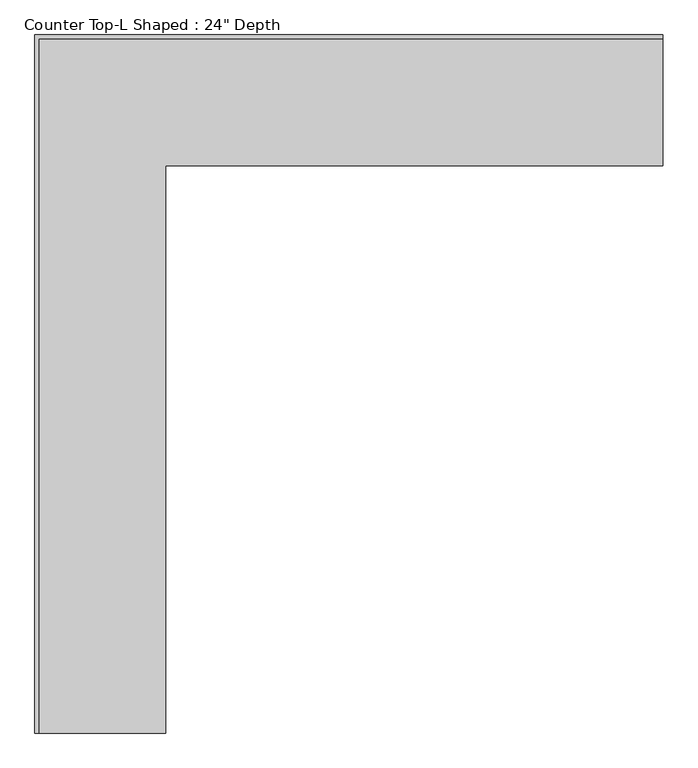
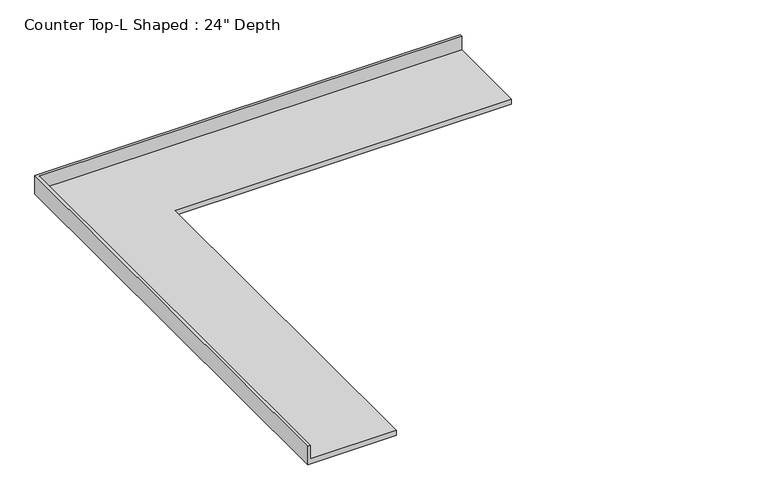
"""IFC4 building model written with IfcOpenShell, lengths in millimetres: furniture geometry."""

from ifc_helpers import new_model, si_unit, origin, place, context, project, spatial, faceted_brep, source, transform, mapped, element, save


def furniture_2797bbf7(model_context):
    return source(origin(), model_context, "Body", "Brep", [
        faceted_brep([(-565.4622951, -3387.4293744, 914.4), (-565.4622951, -635.0, 914.4), (1847.5377049, -635.0, 914.4), (1847.5377049, -19.05, 914.4), (-1181.4122951, -19.05, 914.4), (-1181.4122951, -3387.4293744, 914.4), (1847.5377049, 0.0, 876.3), (1847.5377049, -635.0, 876.3), (-565.4622951, -635.0, 876.3), (-565.4622951, -3387.4293744, 876.3), (-1200.4622951, -3387.4293744, 876.3), (-1200.4622951, 0.0, 876.3), (-1200.4622951, 0.0, 1016.0), (1847.5377049, 0.0, 1016.0), (-1200.4622951, -3387.4293744, 1016.0), (-1181.4122951, -3387.4293744, 1016.0), (1847.5377049, -19.05, 1016.0), (-1181.4122951, -19.05, 1016.0)], [[[0, 1, 2, 3, 4, 5]], [[6, 7, 8, 9, 10, 11]], [[6, 11, 12, 13]], [[11, 10, 14, 12]], [[14, 10, 9, 0, 5, 15]], [[1, 0, 9, 8]], [[2, 1, 8, 7]], [[7, 6, 13, 16, 3, 2]], [[12, 14, 15, 17, 16, 13]], [[3, 16, 17, 4]], [[17, 15, 5, 4]]]),
    ])


if __name__ == "__main__":
    model = new_model("IFC4")
    model_context = context("Model", 3, world=origin())
    ifc_project = project(units=[si_unit("LENGTHUNIT", "METRE", prefix="MILLI")], contexts=[model_context])
    site = spatial("IfcSite", under=ifc_project)
    building = spatial("IfcBuilding", under=site)
    placement = place(None, origin())
    furniture_shape = furniture_2797bbf7(model_context)
    element("IfcFurniture", 1, ObjectType="Counter Top-L Shaped : 24\" Depth", at=placement, inside=building, context=model_context, shape_type="MappedRepresentation", body=[
        mapped(furniture_shape, transform((0.0, 0.0, 0.0), x_axis=(1.0, 0.0, 0.0), y_axis=(0.0, 1.0, 0.0), z_axis=(0.0, 0.0, 1.0))),
    ])
    save(model, "model.ifc")

# Revit data of these elements
# Type "Counter Top-L Shaped : 24\" Depth"
#   Assembly Code = "C1030400"
#   Counter Thickness = 0' - 1 1/2"
#   Depth = 2' - 1"
#   Height = 3' - 0"
#   Length - Leg 1 [instance default] = 8' - 0"
#   Length - Leg 2 [instance default] = 6' - 0"
#   Counter Top Material = none
#   Default Elevation = 0
# Element 1 (IfcFurniture, "Counter Top-L Shaped : 24\" Depth")
#   Length - Leg 1 = 10' - 0"
#   Length - Leg 2 = 11' - 1.36336"
#   Materials on its faces: "Counter Top"
# Materials
#   "Counter Top": class "Wood", colour RGB 226 177 128, transparency 0
